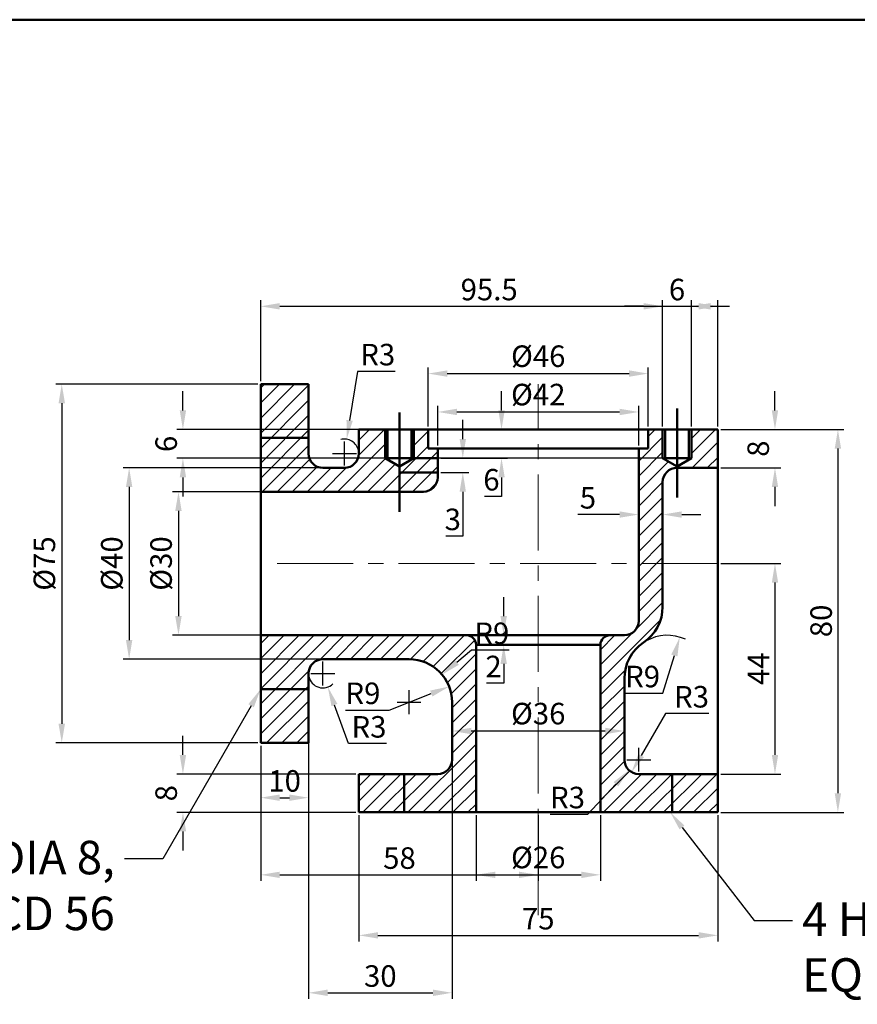
# Model space of a CAD drawing. Units: millimetres. Extents: x -166 to 681, y -4360 to 126.
# Tile 4 of 7: x -22 to 153, y -80 to 126. Entities that reach past the tile are written whole.
import ezdxf
from ezdxf import colors
from ezdxf.entities.mleader import LeaderData, LeaderLine
from ezdxf.math import Vec2, Vec3

# ---------------------------------------------------------------- set-up
doc = ezdxf.new("R2010")
doc.units = ezdxf.units.MM
doc.header["$LTSCALE"] = 0.5
doc.linetypes.add('CENTER', pattern=[50.8, 31.75, -6.35, 6.35, -6.35])
for name, color, linetype, lineweight in [('M-CNTR', 1, 'CENTER', 18), ('M-DIMS', 2, 'Continuous', 25), ('M-HATC', 8, 'Continuous', 18), ('M-OUTL', 7, 'Continuous', 50), ('M-TEXT', 7, 'Continuous', 25), ('M-TTLB', 7, 'Continuous', 50)]:
    doc.layers.add(name, color=color, linetype=linetype, lineweight=lineweight)
doc.styles.get("Standard").update_dxf_attribs({"font": 'arial.ttf'})
doc.dimstyles.new('ISO-25', dxfattribs={"dimtxt": 4.5, "dimasz": 4, "dimexe": 1.25, "dimexo": 0.625, "dimtad": 1, "dimtoh": 1, "dimdec": 1, "dimtxsty": 'Standard', "dimcen": 2.5, "dimadec": 0, "dimazin": 0, "dimtfac": 1, "dimtdec": 1, "dimtofl": 0, "dimtmove": 0, "dimatfit": 3, "dimfxl": 1, "dimarcsym": 0})
pattern_1 = [(45, (-558537.9113, -290104.013), (-1.571544821, 1.571544821), [])]

# ---------------------------------------------------------------- blocks, each defined once
blk = doc.blocks.new('*D1')
at = {"layer": 'Defpoints', "color": 0, "transparency": 16777216}
for p in [(49.3, -39.56), (124.3, -39.56), (124.3, -65.27)]:
    blk.add_point(p, dxfattribs=at)
at = {"layer": 'M-DIMS', "color": 0, "lineweight": -2, "transparency": 16777216}
for p, q in [((49.3, -40.18), (49.3, -66.52)), ((124.3, -40.18), (124.3, -66.52)), ((53.3, -65.27), (120.3, -65.27))]:
    blk.add_line(p, q, dxfattribs=at)
at = {"layer": 'M-DIMS', "color": 0, "transparency": 16777216}
for points in [[(53.3, -64.6), (53.3, -65.94), (49.3, -65.27)], [(120.3, -64.6), (120.3, -65.94), (124.3, -65.27)]]:
    blk.add_solid(points, dxfattribs=at)
at = {"layer": 'M-DIMS', "color": 0, "transparency": 16777216, "insert": (86.8, -62.36), "char_height": 4.5, "attachment_point": 5}
blk.add_mtext('75', dxfattribs=at)
blk = doc.blocks.new('*D2')
at = {"layer": 'Defpoints', "color": 0, "transparency": 16777216}
for p in [(73.8, -39.56), (99.8, -39.56), (99.8, -52.62)]:
    blk.add_point(p, dxfattribs=at)
at = {"layer": 'M-DIMS', "color": 0, "lineweight": -2, "transparency": 16777216}
for p, q in [((73.8, -40.18), (73.8, -53.87)), ((99.8, -40.18), (99.8, -53.87)), ((77.8, -52.62), (95.8, -52.62))]:
    blk.add_line(p, q, dxfattribs=at)
at = {"layer": 'M-DIMS', "color": 0, "transparency": 16777216}
for points in [[(77.8, -51.96), (77.8, -53.29), (73.8, -52.62)], [(95.8, -51.96), (95.8, -53.29), (99.8, -52.62)]]:
    blk.add_solid(points, dxfattribs=at)
at = {"layer": 'M-DIMS', "color": 0, "transparency": 16777216, "insert": (86.8, -49.58), "char_height": 4.5, "attachment_point": 5}
blk.add_mtext('%%C26', dxfattribs=at)
blk = doc.blocks.new('*D3')
at = {"layer": 'Defpoints', "color": 0, "transparency": 16777216}
for p in [(28.8, -25.06), (86.8, -39.56), (86.8, -52.62)]:
    blk.add_point(p, dxfattribs=at)
at = {"layer": 'M-DIMS', "color": 0, "lineweight": -2, "transparency": 16777216}
for p, q in [((28.8, -25.68), (28.8, -53.87)), ((86.8, -40.18), (86.8, -53.87)), ((32.8, -52.62), (82.8, -52.62))]:
    blk.add_line(p, q, dxfattribs=at)
at = {"layer": 'M-DIMS', "color": 0, "transparency": 16777216}
for points in [[(32.8, -51.96), (32.8, -53.29), (28.8, -52.62)], [(82.8, -51.96), (82.8, -53.29), (86.8, -52.62)]]:
    blk.add_solid(points, dxfattribs=at)
at = {"layer": 'M-DIMS', "color": 0, "transparency": 16777216, "insert": (57.8, -49.7), "char_height": 4.5, "attachment_point": 5}
blk.add_mtext('58', dxfattribs=at)
blk = doc.blocks.new('*D4')
at = {"layer": 'Defpoints', "color": 0, "transparency": 16777216}
for p in [(28.8, -25.06), (38.8, -25.06), (38.8, -36.5)]:
    blk.add_point(p, dxfattribs=at)
at = {"layer": 'M-DIMS', "color": 0, "lineweight": -2, "transparency": 16777216}
for p, q in [((28.8, -25.68), (28.8, -37.75)), ((38.8, -25.68), (38.8, -37.75)), ((32.8, -36.5), (34.8, -36.5))]:
    blk.add_line(p, q, dxfattribs=at)
at = {"layer": 'M-DIMS', "color": 0, "transparency": 16777216}
for points in [[(32.8, -35.83), (32.8, -37.17), (28.8, -36.5)], [(34.8, -35.83), (34.8, -37.17), (38.8, -36.5)]]:
    blk.add_solid(points, dxfattribs=at)
at = {"layer": 'M-DIMS', "color": 0, "transparency": 16777216, "insert": (33.8, -33.58), "char_height": 4.5, "attachment_point": 5}
blk.add_mtext('10', dxfattribs=at)
blk = doc.blocks.new('*D5')
at = {"layer": 'Defpoints', "color": 0, "transparency": 16777216}
for p in [(68.8, -22.56), (104.8, -22.56), (104.8, -22.56)]:
    blk.add_point(p, dxfattribs=at)
at = {"layer": 'M-DIMS', "color": 0, "lineweight": -2, "transparency": 16777216}
for p, q in [((68.8, -21.93), (68.8, -21.31)), ((72.8, -22.56), (100.8, -22.56)), ((104.8, -21.93), (104.8, -21.31))]:
    blk.add_line(p, q, dxfattribs=at)
at = {"layer": 'M-DIMS', "color": 0, "transparency": 16777216}
for points in [[(72.8, -21.89), (72.8, -23.23), (68.8, -22.56)], [(100.8, -21.89), (100.8, -23.23), (104.8, -22.56)]]:
    blk.add_solid(points, dxfattribs=at)
at = {"layer": 'M-DIMS', "color": 0, "transparency": 16777216, "insert": (86.8, -19.51), "char_height": 4.5, "attachment_point": 5}
blk.add_mtext('%%C36', dxfattribs=at)
blk = doc.blocks.new('*D6')
at = {"layer": 'Defpoints', "color": 0, "ltscale": 0.5, "transparency": 16777216}
for p in [(28.8, 49.94), (-12.77, -25.06), (28.8, -25.06)]:
    blk.add_point(p, dxfattribs=at)
at = {"layer": 'M-DIMS', "color": 0, "lineweight": -2, "ltscale": 0.5, "transparency": 16777216}
for p, q in [((28.18, 49.94), (-14.02, 49.94)), ((-12.77, 45.94), (-12.77, -21.06)), ((28.18, -25.06), (-14.02, -25.06))]:
    blk.add_line(p, q, dxfattribs=at)
at = {"layer": 'M-DIMS', "color": 0, "ltscale": 0.5, "transparency": 16777216}
for points in [[(-13.44, 45.94), (-12.1, 45.94), (-12.77, 49.94)], [(-13.44, -21.06), (-12.1, -21.06), (-12.77, -25.06)]]:
    blk.add_solid(points, dxfattribs=at)
at = {"layer": 'M-DIMS', "color": 0, "ltscale": 0.5, "transparency": 16777216, "insert": (-15.82, 12.44), "char_height": 4.5, "attachment_point": 5, "rotation": 90}
blk.add_mtext('%%C75', dxfattribs=at)
blk = doc.blocks.new('*D7')
at = {"layer": 'Defpoints', "color": 0, "ltscale": 0.5, "transparency": 16777216}
for p in [(44.05, 32.44), (1.31, -7.56), (44.05, -7.56)]:
    blk.add_point(p, dxfattribs=at)
at = {"layer": 'M-DIMS', "color": 0, "lineweight": -2, "ltscale": 0.5, "transparency": 16777216}
for p, q in [((43.43, 32.44), (0.06, 32.44)), ((1.31, 28.44), (1.31, -3.56)), ((43.43, -7.56), (0.06, -7.56))]:
    blk.add_line(p, q, dxfattribs=at)
at = {"layer": 'M-DIMS', "color": 0, "ltscale": 0.5, "transparency": 16777216}
for points in [[(0.65, 28.44), (1.98, 28.44), (1.31, 32.44)], [(0.65, -3.56), (1.98, -3.56), (1.31, -7.56)]]:
    blk.add_solid(points, dxfattribs=at)
at = {"layer": 'M-DIMS', "color": 0, "ltscale": 0.5, "transparency": 16777216, "insert": (-1.73, 12.44), "char_height": 4.5, "attachment_point": 5, "rotation": 90}
blk.add_mtext('%%C40', dxfattribs=at)
blk = doc.blocks.new('*D8')
at = {"layer": 'Defpoints', "color": 0, "ltscale": 0.5, "transparency": 16777216}
for p in [(45.8, 27.44), (11.62, -2.56), (45.8, -2.56)]:
    blk.add_point(p, dxfattribs=at)
at = {"layer": 'M-DIMS', "color": 0, "lineweight": -2, "ltscale": 0.5, "transparency": 16777216}
for p, q in [((45.18, 27.44), (10.37, 27.44)), ((11.62, 23.44), (11.62, 1.44)), ((45.18, -2.56), (10.37, -2.56))]:
    blk.add_line(p, q, dxfattribs=at)
at = {"layer": 'M-DIMS', "color": 0, "ltscale": 0.5, "transparency": 16777216}
for points in [[(10.95, 23.44), (12.28, 23.44), (11.62, 27.44)], [(10.95, 1.44), (12.28, 1.44), (11.62, -2.56)]]:
    blk.add_solid(points, dxfattribs=at)
at = {"layer": 'M-DIMS', "color": 0, "ltscale": 0.5, "transparency": 16777216, "insert": (8.57, 12.44), "char_height": 4.5, "attachment_point": 5, "rotation": 90}
blk.add_mtext('%%C30', dxfattribs=at)
blk = doc.blocks.new('*D9')
at = {"layer": 'Defpoints', "color": 0, "ltscale": 0.5, "transparency": 16777216}
for p in [(109.8, 52.13), (63.8, 40.44), (109.8, 40.44)]:
    blk.add_point(p, dxfattribs=at)
at = {"layer": 'M-DIMS', "color": 0, "lineweight": -2, "ltscale": 0.5, "transparency": 16777216}
for p, q in [((63.8, 41.07), (63.8, 53.38)), ((67.8, 52.13), (105.8, 52.13)), ((109.8, 41.07), (109.8, 53.38))]:
    blk.add_line(p, q, dxfattribs=at)
at = {"layer": 'M-DIMS', "color": 0, "ltscale": 0.5, "transparency": 16777216}
for points in [[(67.8, 52.8), (67.8, 51.47), (63.8, 52.13)], [(105.8, 52.8), (105.8, 51.47), (109.8, 52.13)]]:
    blk.add_solid(points, dxfattribs=at)
at = {"layer": 'M-DIMS', "color": 0, "ltscale": 0.5, "transparency": 16777216, "insert": (86.8, 55.18), "char_height": 4.5, "attachment_point": 5}
blk.add_mtext('%%C46', dxfattribs=at)
blk = doc.blocks.new('*D10')
at = {"layer": 'Defpoints', "color": 0, "ltscale": 0.5, "transparency": 16777216}
for p in [(107.8, 44.11), (65.8, 36.44), (107.8, 36.44)]:
    blk.add_point(p, dxfattribs=at)
at = {"layer": 'M-DIMS', "color": 0, "lineweight": -2, "ltscale": 0.5, "transparency": 16777216}
for p, q in [((65.8, 37.07), (65.8, 45.36)), ((107.8, 37.07), (107.8, 45.36)), ((69.8, 44.11), (103.8, 44.11))]:
    blk.add_line(p, q, dxfattribs=at)
at = {"layer": 'M-DIMS', "color": 0, "ltscale": 0.5, "transparency": 16777216}
for points in [[(69.8, 44.78), (69.8, 43.44), (65.8, 44.11)], [(103.8, 44.78), (103.8, 43.44), (107.8, 44.11)]]:
    blk.add_solid(points, dxfattribs=at)
at = {"layer": 'M-DIMS', "color": 0, "ltscale": 0.5, "transparency": 16777216, "insert": (86.8, 47.16), "char_height": 4.5, "attachment_point": 5}
blk.add_mtext('%%C42', dxfattribs=at)
blk = doc.blocks.new('*D11')
at = {"layer": 'Defpoints', "color": 0, "ltscale": 0.5, "transparency": 16777216}
for p in [(124.3, 12.44), (124.3, -31.56), (136.27, -31.56)]:
    blk.add_point(p, dxfattribs=at)
at = {"layer": 'M-DIMS', "color": 0, "lineweight": -2, "ltscale": 0.5, "transparency": 16777216}
for p, q in [((124.93, 12.44), (137.52, 12.44)), ((136.27, 8.44), (136.27, -27.56)), ((124.93, -31.56), (137.52, -31.56))]:
    blk.add_line(p, q, dxfattribs=at)
at = {"layer": 'M-DIMS', "color": 0, "ltscale": 0.5, "transparency": 16777216}
for points in [[(135.61, 8.44), (136.94, 8.44), (136.27, 12.44)], [(135.61, -27.56), (136.94, -27.56), (136.27, -31.56)]]:
    blk.add_solid(points, dxfattribs=at)
at = {"layer": 'M-DIMS', "color": 0, "ltscale": 0.5, "transparency": 16777216, "insert": (133.4, -9.56), "char_height": 4.5, "attachment_point": 5, "rotation": 90}
blk.add_mtext('44', dxfattribs=at)
blk = doc.blocks.new('*D12')
at = {"layer": 'Defpoints', "color": 0, "ltscale": 0.5, "transparency": 16777216}
for p in [(124.3, 40.44), (124.3, 32.44), (136.27, 32.44)]:
    blk.add_point(p, dxfattribs=at)
at = {"layer": 'M-DIMS', "color": 0, "lineweight": -2, "ltscale": 0.5, "transparency": 16777216}
for p, q in [((136.27, 44.44), (136.27, 48.44)), ((124.93, 40.44), (137.52, 40.44)), ((124.93, 32.44), (137.52, 32.44)), ((136.27, 28.44), (136.27, 24.44))]:
    blk.add_line(p, q, dxfattribs=at)
at = {"layer": 'M-DIMS', "color": 0, "ltscale": 0.5, "transparency": 16777216}
for points in [[(135.61, 44.44), (136.94, 44.44), (136.27, 40.44)], [(135.61, 28.44), (136.94, 28.44), (136.27, 32.44)]]:
    blk.add_solid(points, dxfattribs=at)
at = {"layer": 'M-DIMS', "color": 0, "ltscale": 0.5, "transparency": 16777216, "insert": (133.35, 36.44), "char_height": 4.5, "attachment_point": 5, "rotation": 90}
blk.add_mtext('8', dxfattribs=at)
blk = doc.blocks.new('*D13')
at = {"layer": 'Defpoints', "color": 0, "ltscale": 0.5, "transparency": 16777216}
for p in [(124.3, 40.44), (124.3, -39.56), (149.42, -39.56)]:
    blk.add_point(p, dxfattribs=at)
at = {"layer": 'M-DIMS', "color": 0, "lineweight": -2, "ltscale": 0.5, "transparency": 16777216}
for p, q in [((124.93, 40.44), (150.67, 40.44)), ((149.42, 36.44), (149.42, -35.56)), ((124.93, -39.56), (150.67, -39.56))]:
    blk.add_line(p, q, dxfattribs=at)
at = {"layer": 'M-DIMS', "color": 0, "ltscale": 0.5, "transparency": 16777216}
for points in [[(148.75, 36.44), (150.09, 36.44), (149.42, 40.44)], [(148.75, -35.56), (150.09, -35.56), (149.42, -39.56)]]:
    blk.add_solid(points, dxfattribs=at)
at = {"layer": 'M-DIMS', "color": 0, "ltscale": 0.5, "transparency": 16777216, "insert": (146.5, 0.44), "char_height": 4.5, "attachment_point": 5, "rotation": 90}
blk.add_mtext('80', dxfattribs=at)
blk = doc.blocks.new('*D14')
at = {"layer": 'Defpoints', "color": 0, "ltscale": 0.5, "transparency": 16777216}
for p in [(112.8, 22.67), (107.8, 22.01), (112.8, 22.01)]:
    blk.add_point(p, dxfattribs=at)
at = {"layer": 'M-DIMS', "color": 0, "lineweight": -2, "ltscale": 0.5, "transparency": 16777216}
for p, q in [((103.8, 22.67), (95.07, 22.67)), ((107.8, 22.63), (107.8, 23.92)), ((112.8, 22.63), (112.8, 23.92)), ((116.8, 22.67), (120.8, 22.67))]:
    blk.add_line(p, q, dxfattribs=at)
at = {"layer": 'M-DIMS', "color": 0, "ltscale": 0.5, "transparency": 16777216}
for points in [[(103.8, 23.34), (103.8, 22.01), (107.8, 22.67)], [(116.8, 23.34), (116.8, 22.01), (112.8, 22.67)]]:
    blk.add_solid(points, dxfattribs=at)
at = {"layer": 'M-DIMS', "color": 0, "ltscale": 0.5, "transparency": 16777216, "insert": (97.19, 25.59), "char_height": 4.5, "attachment_point": 5}
blk.add_mtext('5', dxfattribs=at)
blk = doc.blocks.new('*D15')
at = {"layer": 'Defpoints', "color": 0, "ltscale": 0.5, "transparency": 16777216}
for p in [(65.8, 34.44), (65.8, 31.44), (71.04, 31.44)]:
    blk.add_point(p, dxfattribs=at)
at = {"layer": 'M-DIMS', "color": 0, "lineweight": -2, "ltscale": 0.5, "transparency": 16777216}
for p, q in [((71.04, 38.44), (71.04, 42.44)), ((66.43, 34.44), (72.29, 34.44)), ((66.43, 31.44), (72.29, 31.44)), ((71.04, 27.44), (71.04, 18.16)), ((71.04, 18.16), (67.46, 18.16))]:
    blk.add_line(p, q, dxfattribs=at)
at = {"layer": 'M-DIMS', "color": 0, "ltscale": 0.5, "transparency": 16777216}
for points in [[(70.37, 38.44), (71.7, 38.44), (71.04, 34.44)], [(70.37, 27.44), (71.7, 27.44), (71.04, 31.44)]]:
    blk.add_solid(points, dxfattribs=at)
at = {"layer": 'M-DIMS', "color": 0, "ltscale": 0.5, "transparency": 16777216, "insert": (68.94, 21.08), "char_height": 4.5, "attachment_point": 5}
blk.add_mtext('3', dxfattribs=at)
blk = doc.blocks.new('*D16')
at = {"layer": 'Defpoints', "color": 0, "ltscale": 0.5, "transparency": 16777216}
for p in [(65.8, 40.44), (65.8, 34.44), (79.13, 34.44)]:
    blk.add_point(p, dxfattribs=at)
at = {"layer": 'M-DIMS', "color": 0, "lineweight": -2, "ltscale": 0.5, "transparency": 16777216}
for p, q in [((79.13, 44.44), (79.13, 48.44)), ((66.43, 40.44), (80.38, 40.44)), ((66.43, 34.44), (80.38, 34.44)), ((79.13, 30.44), (79.13, 26.44)), ((79.13, 26.44), (75.54, 26.44))]:
    blk.add_line(p, q, dxfattribs=at)
at = {"layer": 'M-DIMS', "color": 0, "ltscale": 0.5, "transparency": 16777216}
for points in [[(78.47, 44.44), (79.8, 44.44), (79.13, 40.44)], [(78.47, 30.44), (79.8, 30.44), (79.13, 34.44)]]:
    blk.add_solid(points, dxfattribs=at)
at = {"layer": 'M-DIMS', "color": 0, "ltscale": 0.5, "transparency": 16777216, "insert": (77.02, 29.36), "char_height": 4.5, "attachment_point": 5}
blk.add_mtext('6', dxfattribs=at)
blk = doc.blocks.new('*D17')
at = {"layer": 'Defpoints', "color": 0, "ltscale": 0.5, "transparency": 16777216}
for p in [(77.02, -2.56), (77.02, -4.56), (79.58, -4.56)]:
    blk.add_point(p, dxfattribs=at)
at = {"layer": 'M-DIMS', "color": 0, "lineweight": -2, "ltscale": 0.5, "transparency": 16777216}
for p, q in [((79.58, 1.44), (79.58, 5.44)), ((77.65, -2.56), (80.83, -2.56)), ((77.65, -4.56), (80.83, -4.56)), ((79.58, -8.56), (79.58, -12.56)), ((79.58, -12.56), (75.97, -12.56))]:
    blk.add_line(p, q, dxfattribs=at)
at = {"layer": 'M-DIMS', "color": 0, "ltscale": 0.5, "transparency": 16777216}
for points in [[(78.91, 1.44), (80.25, 1.44), (79.58, -2.56)], [(78.91, -8.56), (80.25, -8.56), (79.58, -4.56)]]:
    blk.add_solid(points, dxfattribs=at)
at = {"layer": 'M-DIMS', "color": 0, "ltscale": 0.5, "transparency": 16777216, "insert": (77.46, -9.67), "char_height": 4.5, "attachment_point": 5}
blk.add_mtext('2', dxfattribs=at)
blk = doc.blocks.new('*D18')
at = {"layer": 'Defpoints', "color": 0, "ltscale": 0.5, "transparency": 16777216}
for p in [(41.8, -10.56), (42.83, -13.38)]:
    blk.add_point(p, dxfattribs=at)
at = {"layer": 'M-DIMS', "color": 0, "lineweight": -2, "ltscale": 0.5, "transparency": 16777216}
for p, q in [((41.8, -13.06), (41.8, -8.06)), ((39.3, -10.56), (44.3, -10.56)), ((47.17, -25.2), (44.21, -17.13)), ((55.06, -25.2), (47.17, -25.2))]:
    blk.add_line(p, q, dxfattribs=at)
blk.add_arc((41.8, -10.56), 3, 191.9366, 314.026, dxfattribs=at)
at = {"layer": 'M-DIMS', "color": 0, "ltscale": 0.5, "transparency": 16777216}
blk.add_solid([(44.84, -16.9), (43.59, -17.36), (42.83, -13.38)], dxfattribs=at)
at = {"layer": 'M-DIMS', "color": 0, "ltscale": 0.5, "transparency": 16777216, "insert": (51.43, -22.28), "char_height": 4.5, "attachment_point": 5}
blk.add_mtext('R3', dxfattribs=at)
blk = doc.blocks.new('*D19')
at = {"layer": 'Defpoints', "color": 0, "ltscale": 0.5, "transparency": 16777216}
for p in [(68.18, -13.27), (59.8, -16.56)]:
    blk.add_point(p, dxfattribs=at)
at = {"layer": 'M-DIMS', "color": 0, "lineweight": -2, "ltscale": 0.5, "transparency": 16777216}
for p, q in [((55.64, -18.19), (64.46, -14.73)), ((46.54, -18.19), (55.64, -18.19))]:
    blk.add_line(p, q, dxfattribs=at)
at = {"layer": 'M-DIMS', "color": 0, "ltscale": 0.5, "transparency": 16777216}
blk.add_solid([(64.21, -14.11), (64.7, -15.35), (68.18, -13.27)], dxfattribs=at)
at = {"layer": 'M-DIMS', "color": 0, "ltscale": 0.5, "transparency": 16777216, "insert": (50.17, -15.27), "char_height": 4.5, "attachment_point": 5}
blk.add_mtext('R9', dxfattribs=at)
blk = doc.blocks.new('*D20')
at = {"layer": 'Defpoints', "color": 0, "ltscale": 0.5, "transparency": 16777216}
for p in [(107.8, -28.56), (106.3, -31.16)]:
    blk.add_point(p, dxfattribs=at)
at = {"layer": 'M-DIMS', "color": 0, "lineweight": -2, "ltscale": 0.5, "transparency": 16777216}
for p, q in [((113.37, -18.92), (108.3, -27.69)), ((122.46, -18.92), (113.37, -18.92))]:
    blk.add_line(p, q, dxfattribs=at)
at = {"layer": 'M-DIMS', "color": 0, "ltscale": 0.5, "transparency": 16777216}
blk.add_solid([(107.72, -27.36), (108.88, -28.03), (106.3, -31.16)], dxfattribs=at)
at = {"layer": 'M-DIMS', "color": 0, "ltscale": 0.5, "transparency": 16777216, "insert": (118.83, -15.99), "char_height": 4.5, "attachment_point": 5}
blk.add_mtext('R3', dxfattribs=at)
blk = doc.blocks.new('*D21')
at = {"layer": 'Defpoints', "color": 0, "ltscale": 0.5, "transparency": 16777216}
for p in [(116.39, -2.94), (113.8, -11.56)]:
    blk.add_point(p, dxfattribs=at)
at = {"layer": 'M-DIMS', "color": 0, "lineweight": -2, "ltscale": 0.5, "transparency": 16777216}
for p, q in [((112.86, -14.68), (115.24, -6.77)), ((104.97, -14.68), (112.86, -14.68))]:
    blk.add_line(p, q, dxfattribs=at)
blk.add_arc((113.8, -11.56), 9, 65.3168, 119.7701, dxfattribs=at)
at = {"layer": 'M-DIMS', "color": 0, "ltscale": 0.5, "transparency": 16777216}
blk.add_solid([(114.6, -6.58), (115.88, -6.96), (116.39, -2.94)], dxfattribs=at)
at = {"layer": 'M-DIMS', "color": 0, "ltscale": 0.5, "transparency": 16777216, "insert": (108.61, -11.76), "char_height": 4.5, "attachment_point": 5}
blk.add_mtext('R9', dxfattribs=at)
blk = doc.blocks.new('*D22')
at = {"layer": 'Defpoints', "color": 0, "ltscale": 0.5, "transparency": 16777216}
for p in [(46.77, 38.4), (46.3, 35.44)]:
    blk.add_point(p, dxfattribs=at)
at = {"layer": 'M-DIMS', "color": 0, "lineweight": -2, "ltscale": 0.5, "transparency": 16777216}
for p, q in [((49.01, 52.58), (47.39, 42.36)), ((56.89, 52.58), (49.01, 52.58)), ((46.3, 32.94), (46.3, 37.94)), ((43.8, 35.44), (48.8, 35.44))]:
    blk.add_line(p, q, dxfattribs=at)
blk.add_arc((46.3, 35.44), 3, 11.9366, 104.8944, dxfattribs=at)
at = {"layer": 'M-DIMS', "color": 0, "ltscale": 0.5, "transparency": 16777216}
blk.add_solid([(46.73, 42.46), (48.05, 42.25), (46.77, 38.4)], dxfattribs=at)
at = {"layer": 'M-DIMS', "color": 0, "ltscale": 0.5, "transparency": 16777216, "insert": (53.26, 55.51), "char_height": 4.5, "attachment_point": 5}
blk.add_mtext('R3', dxfattribs=at)
blk = doc.blocks.new('*D74')
at = {"layer": 'Defpoints', "color": 0, "ltscale": 0.5, "transparency": 16777216}
for p in [(124.3, 66.19), (28.8, 49.94), (124.3, 40.44)]:
    blk.add_point(p, dxfattribs=at)
at = {"layer": 'M-DIMS', "color": 0, "lineweight": -2, "ltscale": 0.5, "transparency": 16777216}
for p, q in [((28.8, 50.57), (28.8, 67.44)), ((32.8, 66.19), (120.3, 66.19)), ((124.3, 41.07), (124.3, 67.44))]:
    blk.add_line(p, q, dxfattribs=at)
at = {"layer": 'M-DIMS', "color": 0, "ltscale": 0.5, "transparency": 16777216}
for points in [[(32.8, 66.86), (32.8, 65.52), (28.8, 66.19)], [(120.3, 66.86), (120.3, 65.52), (124.3, 66.19)]]:
    blk.add_solid(points, dxfattribs=at)
at = {"layer": 'M-DIMS', "color": 0, "ltscale": 0.5, "transparency": 16777216, "insert": (76.55, 69.11), "char_height": 4.5, "attachment_point": 5}
blk.add_mtext('95.5', dxfattribs=at)
blk = doc.blocks.new('*D75')
at = {"layer": 'Defpoints', "color": 0, "ltscale": 0.5, "transparency": 16777216}
for p in [(12.55, -31.56), (49.3, -31.56), (49.3, -39.56)]:
    blk.add_point(p, dxfattribs=at)
at = {"layer": 'M-DIMS', "color": 0, "lineweight": -2, "ltscale": 0.5, "transparency": 16777216}
for p, q in [((12.55, -27.56), (12.55, -23.56)), ((48.68, -31.56), (11.3, -31.56)), ((48.68, -39.56), (11.3, -39.56)), ((12.55, -43.56), (12.55, -47.56))]:
    blk.add_line(p, q, dxfattribs=at)
at = {"layer": 'M-DIMS', "color": 0, "ltscale": 0.5, "transparency": 16777216}
for points in [[(11.88, -27.56), (13.22, -27.56), (12.55, -31.56)], [(11.88, -43.56), (13.22, -43.56), (12.55, -39.56)]]:
    blk.add_solid(points, dxfattribs=at)
at = {"layer": 'M-DIMS', "color": 0, "ltscale": 0.5, "transparency": 16777216, "insert": (9.63, -35.56), "char_height": 4.5, "attachment_point": 5, "rotation": 90}
blk.add_mtext('8', dxfattribs=at)
blk = doc.blocks.new('*D76')
at = {"layer": 'Defpoints', "color": 0, "ltscale": 0.5, "transparency": 16777216}
for p in [(118.8, 66.19), (112.8, 40.44), (118.8, 40.44)]:
    blk.add_point(p, dxfattribs=at)
at = {"layer": 'M-DIMS', "color": 0, "lineweight": -2, "ltscale": 0.5, "transparency": 16777216}
for p, q in [((108.8, 66.19), (104.8, 66.19)), ((112.8, 41.07), (112.8, 67.44)), ((118.8, 41.07), (118.8, 67.44)), ((122.8, 66.19), (126.8, 66.19))]:
    blk.add_line(p, q, dxfattribs=at)
at = {"layer": 'M-DIMS', "color": 0, "ltscale": 0.5, "transparency": 16777216}
for points in [[(108.8, 66.86), (108.8, 65.52), (112.8, 66.19)], [(122.8, 66.86), (122.8, 65.52), (118.8, 66.19)]]:
    blk.add_solid(points, dxfattribs=at)
at = {"layer": 'M-DIMS', "color": 0, "ltscale": 0.5, "transparency": 16777216, "insert": (115.8, 69.11), "char_height": 4.5, "attachment_point": 5}
blk.add_mtext('6', dxfattribs=at)
blk = doc.blocks.new('*D77')
at = {"layer": 'Defpoints', "color": 0, "ltscale": 0.5, "transparency": 16777216}
for p in [(118.8, 40.44), (12.55, 34.44), (118.8, 34.44)]:
    blk.add_point(p, dxfattribs=at)
at = {"layer": 'M-DIMS', "color": 0, "lineweight": -2, "ltscale": 0.5, "transparency": 16777216}
for p, q in [((12.55, 44.44), (12.55, 48.44)), ((118.18, 40.44), (11.3, 40.44)), ((118.18, 34.44), (11.3, 34.44)), ((12.55, 30.44), (12.55, 26.44))]:
    blk.add_line(p, q, dxfattribs=at)
at = {"layer": 'M-DIMS', "color": 0, "ltscale": 0.5, "transparency": 16777216}
for points in [[(11.88, 44.44), (13.22, 44.44), (12.55, 40.44)], [(11.88, 30.44), (13.22, 30.44), (12.55, 34.44)]]:
    blk.add_solid(points, dxfattribs=at)
at = {"layer": 'M-DIMS', "color": 0, "ltscale": 0.5, "transparency": 16777216, "insert": (9.63, 37.44), "char_height": 4.5, "attachment_point": 5, "rotation": 90}
blk.add_mtext('6', dxfattribs=at)
blk = doc.blocks.new('*D82')
at = {"layer": 'Defpoints', "color": 0, "ltscale": 0.5, "transparency": 16777216}
for p in [(38.8, -13.81), (68.8, -16.56), (68.8, -77.27)]:
    blk.add_point(p, dxfattribs=at)
at = {"layer": 'M-DIMS', "color": 0, "lineweight": -2, "ltscale": 0.5, "transparency": 16777216}
for p, q in [((38.8, -14.43), (38.8, -78.52)), ((68.8, -17.18), (68.8, -78.52)), ((42.8, -77.27), (64.8, -77.27))]:
    blk.add_line(p, q, dxfattribs=at)
at = {"layer": 'M-DIMS', "color": 0, "ltscale": 0.5, "transparency": 16777216}
for points in [[(42.8, -76.6), (42.8, -77.94), (38.8, -77.27)], [(64.8, -76.6), (64.8, -77.94), (68.8, -77.27)]]:
    blk.add_solid(points, dxfattribs=at)
at = {"layer": 'M-DIMS', "color": 0, "ltscale": 0.5, "transparency": 16777216, "insert": (53.8, -74.35), "char_height": 4.5, "attachment_point": 5}
blk.add_mtext('30', dxfattribs=at)
blk = doc.blocks.new('*D92')
at = {"layer": 'Defpoints', "color": 0, "ltscale": 0.5, "transparency": 16777216}
for p in [(66.7, -10.78), (59.8, -16.56)]:
    blk.add_point(p, dxfattribs=at)
at = {"layer": 'M-DIMS', "color": 0, "lineweight": -2, "ltscale": 0.5, "transparency": 16777216}
for p, q in [((72.84, -5.65), (69.77, -8.22)), ((80.73, -5.65), (72.84, -5.65)), ((59.8, -19.06), (59.8, -14.06)), ((57.3, -16.56), (62.3, -16.56))]:
    blk.add_line(p, q, dxfattribs=at)
at = {"layer": 'M-DIMS', "color": 0, "ltscale": 0.5, "transparency": 16777216}
blk.add_solid([(69.34, -7.7), (70.2, -8.73), (66.7, -10.78)], dxfattribs=at)
at = {"layer": 'M-DIMS', "color": 0, "ltscale": 0.5, "transparency": 16777216, "insert": (77.1, -2.73), "char_height": 4.5, "attachment_point": 5}
blk.add_mtext('R9', dxfattribs=at)
blk = doc.blocks.new('*D93')
at = {"layer": 'Defpoints', "color": 0, "ltscale": 0.5, "transparency": 16777216}
for p in [(107.8, -28.56), (105.76, -30.75)]:
    blk.add_point(p, dxfattribs=at)
at = {"layer": 'M-DIMS', "color": 0, "lineweight": -2, "ltscale": 0.5, "transparency": 16777216}
for p, q in [((107.8, -31.06), (107.8, -26.06)), ((105.3, -28.56), (110.3, -28.56)), ((97.17, -39.97), (103.03, -33.68)), ((89.29, -39.97), (97.17, -39.97))]:
    blk.add_line(p, q, dxfattribs=at)
at = {"layer": 'M-DIMS', "color": 0, "ltscale": 0.5, "transparency": 16777216}
blk.add_solid([(102.54, -33.23), (103.52, -34.14), (105.76, -30.75)], dxfattribs=at)
at = {"layer": 'M-DIMS', "color": 0, "ltscale": 0.5, "transparency": 16777216, "insert": (92.92, -37.05), "char_height": 4.5, "attachment_point": 5}
blk.add_mtext('R3', dxfattribs=at)

msp = doc.modelspace()

# ---------------------------------------------------------------- hatches: boundary and pattern name
at = {"layer": 'M-HATC', "ltscale": 0.5}
h = msp.add_hatch(dxfattribs=at)
h.set_pattern_fill('ANSI31', color=256, scale=0.7)
h.set_pattern_definition(pattern_1)
h.paths.add_polyline_path([(38.8008, 49.9412), (28.8008, 49.9412), (28.8008, 38.6912), (38.8008, 38.6912)])
h.paths.add_polyline_path([(57.8008, 32.7092), (54.8008, 34.4412), (54.8008, 40.4412), (49.3008, 40.4412), (49.3008, 35.4412, -0.41421356), (46.3008, 32.4412), (41.8008, 32.4412, -0.41421356), (38.8008, 35.4412), (38.8008, 38.6912), (28.8008, 38.6912), (28.8008, 27.4412), (57.8008, 27.4412)])
h.paths.add_polyline_path([(65.8008, 34.4412), (60.8008, 34.4412), (57.8008, 32.7092), (57.8008, 31.4412), (65.8008, 31.4412)])
h.paths.add_polyline_path([(65.8008, 30.4412), (65.8008, 31.4412), (57.8008, 31.4412), (57.8008, 27.4412), (62.8008, 27.4412, 0.41421356)])
h.paths.add_polyline_path([(124.3008, 40.4412), (118.8008, 40.4412), (118.8008, 34.4412), (115.8008, 32.7092), (115.8008, 32.4412), (124.3008, 32.4412)])
h.paths.add_polyline_path([(115.8008, 32.7092), (112.8008, 34.4412), (112.8008, 40.4412), (109.8008, 40.4412), (109.8008, 36.4412), (107.8008, 36.4412), (107.8008, 12.4412), (112.8008, 12.4412), (112.8008, 29.4412, -0.41421356), (115.8008, 32.4412)])
h.paths.add_polyline_path([(112.8008, 12.4412), (107.8008, 12.4412), (107.8008, 0.4412, -0.41421356), (104.8008, -2.5588), (101.8008, -2.5588, 0.41421356), (99.8008, -4.5588), (99.8008, -39.5588), (124.3008, -39.5588), (124.3008, -31.5588), (107.8008, -31.5588, -0.41421356), (104.8008, -28.5588), (104.8008, -11.5588, -0.25049165), (108.8008, -4.0754, 0.25049165), (112.8008, 3.4079)])
h.paths.add_polyline_path([(73.8008, -4.5588, 0.41421356), (71.8008, -2.5588), (28.8008, -2.5588), (28.8008, -13.8088), (38.8008, -13.8088), (38.8008, -10.5588, -0.41421356), (41.8008, -7.5588), (59.8008, -7.5588, -0.41421356), (68.8008, -16.5588), (68.8008, -28.5588, -0.41421356), (65.8008, -31.5588), (49.3008, -31.5588), (49.3008, -39.5588), (73.8008, -39.5588)])
h.paths.add_polyline_path([(38.8008, -13.8088), (28.8008, -13.8088), (28.8008, -25.0588), (38.8008, -25.0588)], flags=17)
h = msp.add_hatch(dxfattribs=at)
h.set_pattern_fill('ANSI31', color=256, scale=0.7)
h.set_pattern_definition(pattern_1)
h.paths.add_polyline_path([(63.8008, 40.4412), (60.8008, 40.4412), (60.8008, 34.4412), (65.8008, 34.4412), (65.8008, 36.4412), (63.8008, 36.4412)])

# ---------------------------------------------------------------- linework, layer by layer
at = {"layer": 'M-CNTR'}
for p, q in [((86.8008, -61.0209), (86.8008, 49.9412)), ((124.3008, 12.4412), (28.8008, 12.4412))]:
    msp.add_line(p, q, dxfattribs=at)
at = {"layer": 'M-OUTL'}
for p, q in [((38.8008, 49.9412), (28.8008, 49.9412)), ((28.8008, 27.4412), (28.8008, 49.9412)), ((38.8008, 35.4412), (38.8008, 49.9412)), ((57.8008, 43.9754), (57.8008, 23.2561)), ((115.8008, 44.8622), (115.8008, 26.2478)), ((49.3008, 35.4412), (49.3008, 40.4412)), ((109.8008, 40.4412), (49.3008, 40.4412)), ((54.8008, 40.4412), (54.8008, 34.4412)), ((55.3008, 40.4412), (55.3008, 34.1526)), ((60.3008, 40.4412), (60.3008, 34.1526)), ((60.8008, 40.4412), (60.8008, 34.4412)), ((63.8008, 36.4412), (63.8008, 40.4412)), ((115.8008, 40.4412), (109.8008, 40.4412)), ((109.8008, 36.4412), (109.8008, 40.4412)), ((112.8008, 40.4412), (112.8008, 34.4412)), ((113.3008, 40.4412), (113.3008, 34.1526)), ((124.3008, 40.4412), (115.8008, 40.4412)), ((118.3008, 40.4412), (118.3008, 34.1526)), ((118.8008, 40.4412), (118.8008, 34.4412)), ((124.3008, -31.5588), (124.3008, 40.4412)), ((28.8008, 38.6912), (38.8008, 38.6912)), ((109.8008, 36.4412), (63.8008, 36.4412)), ((65.8008, 30.4412), (65.8008, 36.4412)), ((107.8008, 0.4412), (107.8008, 36.4412)), ((57.8008, 32.7092), (54.8008, 34.4412)), ((60.3008, 34.4412), (55.3008, 34.4412)), ((60.8008, 34.4412), (57.8008, 32.7092)), ((65.8008, 34.4412), (60.8008, 34.4412)), ((112.8008, 34.4412), (115.8008, 32.7092)), ((118.3008, 34.4412), (113.3008, 34.4412)), ((115.8008, 32.7092), (118.8008, 34.4412)), ((46.3008, 32.4412), (41.8008, 32.4412)), ((65.8008, 31.4412), (57.8008, 31.4412)), ((124.3008, 32.4412), (115.8008, 32.4412)), ((112.8008, 3.4079), (112.8008, 29.4412)), ((28.8008, -25.0588), (28.8008, 27.4412)), ((62.8008, 27.4412), (28.8008, 27.4412)), ((71.8008, -2.5588), (28.8008, -2.5588)), ((71.8008, -2.5588), (101.8008, -2.5588)), ((104.8008, -2.5588), (101.8008, -2.5588)), ((73.8008, -39.5588), (73.8008, -4.5588)), ((73.8008, -4.5588), (99.8008, -4.5588)), ((99.8008, -39.5588), (99.8008, -4.5588)), ((59.8008, -7.5588), (41.8008, -7.5588)), ((38.8008, -25.0588), (38.8008, -10.5588)), ((104.8008, -28.5588), (104.8008, -11.5588)), ((28.8008, -13.8088), (38.8008, -13.8088)), ((68.8008, -28.5588), (68.8008, -16.5588)), ((38.8008, -25.0588), (28.8008, -25.0588)), ((49.3008, -31.5588), (49.3008, -39.5588)), ((65.8008, -31.5588), (49.3008, -31.5588)), ((124.3008, -31.5588), (107.8008, -31.5588)), ((124.3008, -39.5588), (124.3008, -31.5588)), ((49.3008, -39.5588), (124.3008, -39.5588))]:
    msp.add_line(p, q, dxfattribs=at)
at = {"layer": 'M-OUTL', "ltscale": 0.5}
for p, q in [((58.8008, -39.5588), (58.8008, -31.5588)), ((114.8008, -39.5588), (114.8008, -31.5588))]:
    msp.add_line(p, q, dxfattribs=at)
at = {"layer": 'M-OUTL'}
for centre, radius, start, end in [((41.8008, 35.4412), 3, 180, 270), ((46.3008, 35.4412), 3, 270, 0), ((115.8008, 29.4412), 3, 90, 180), ((62.8008, 30.4412), 3, 270, 0), ((103.8008, 3.4079), 9, 303.748989, 0), ((104.8008, 0.4412), 3, 270, 0), ((71.8008, -4.5588), 2, 0, 90), ((101.8008, -4.5588), 2, 90, 180), ((113.8008, -11.5588), 9, 123.748989, 180), ((41.8008, -10.5588), 3, 90, 180), ((59.8008, -16.5588), 9, 0, 90), ((65.8008, -28.5588), 3, 270, 0), ((107.8008, -28.5588), 3, 180, 270)]:
    msp.add_arc(centre, radius, start, end, dxfattribs=at)
at = {"layer": 'M-TTLB', "ltscale": 0.5}
msp.add_lwpolyline([(-165.9437, 126.0872), (680.7907, 126.0872), (680.7907, -430.0081), (-165.9437, -430.0081)], close=True, dxfattribs=at)

# ---------------------------------------------------------------- dimensions: what is measured, and where the dimension line sits
at = {"layer": 'M-DIMS', "ltscale": 0.5}
for base, p1, p2, override, picture, middle in [((124.3008, 66.1912), (28.8008, 49.9412), (124.3008, 40.4412), {"dimdec": 1, "dimlfac": 1, "dimrnd": 0, "dimzin": 0, "dimdsep": 46, "dimlunit": 2}, '*D74', (76.5508, 69.1138)), ((118.8008, 66.1912), (112.8008, 40.4412), (118.8008, 40.4412), {"dimdec": 0, "dimlfac": 1, "dimrnd": 0, "dimzin": 0, "dimdsep": 46, "dimlunit": 2}, '*D76', (115.8008, 69.1138)), ((68.8008, -77.2709), (38.8008, -13.8088), (68.8008, -16.5588), {"dimdec": 0, "dimlfac": 1, "dimrnd": 0, "dimzin": 0, "dimdsep": 46, "dimlunit": 2}, '*D82', (53.8008, -74.3467))]:
    dim = msp.add_linear_dim(base=base, p1=p1, p2=p2, dimstyle='ISO-25', override=override, dxfattribs=at)
    dim.commit()
    dim.dimension.update_dxf_attribs({"geometry": picture, "text_midpoint": middle})
for center, mpoint, picture, middle in [((46.3008, 35.4412), (46.769, 38.4045), '*D22', (53.2623, 52.5816)), ((113.8008, -11.5588), (116.3909, -2.9395), '*D21', (108.6054, -14.6788)), ((59.8008, -16.5588), (68.1801, -13.2744), '*D19', (50.1714, -18.1895)), ((107.8008, -28.5588), (106.3008, -31.1568), '*D20', (118.829, -18.9191))]:
    dim = msp.add_radius_dim(center=center, mpoint=mpoint, dimstyle='ISO-25', override={"dimclrd": 0, "dimclre": 0, "dimclrt": 0}, dxfattribs=at)
    dim.commit()
    dim.dimension.update_dxf_attribs({"geometry": picture, "text_midpoint": middle, "dimtype": 164})
for base, p1, p2, picture, middle in [((109.8008, 52.1339), (63.8008, 40.4412), (109.8008, 40.4412), '*D9', (86.8008, 55.1823)), ((107.8008, 44.1105), (65.8008, 36.4412), (107.8008, 36.4412), '*D10', (86.8008, 47.1589))]:
    dim = msp.add_linear_dim(base=base, p1=p1, p2=p2, text='%%C<>', dimstyle='ISO-25', override={"dimclrd": 0, "dimclre": 0, "dimclrt": 0}, dxfattribs=at)
    dim.commit()
    dim.dimension.update_dxf_attribs({"geometry": picture, "text_midpoint": middle})
for base, p1, p2, picture, middle in [((-12.7702, -25.0588), (28.8008, 49.9412), (28.8008, -25.0588), '*D6', (-15.8186, 12.4412)), ((1.3147, -7.5588), (44.0508, 32.4412), (44.0508, -7.5588), '*D7', (-1.7338, 12.4412)), ((11.6155, -2.5588), (45.8008, 27.4412), (45.8008, -2.5588), '*D8', (8.5671, 12.4412))]:
    dim = msp.add_linear_dim(base=base, p1=p1, p2=p2, angle=90, text='%%C<>', dimstyle='ISO-25', override={"dimclrd": 0, "dimclre": 0, "dimclrt": 0}, dxfattribs=at)
    dim.commit()
    dim.dimension.update_dxf_attribs({"geometry": picture, "text_midpoint": middle})
for base, p1, p2, override, picture, middle in [((12.5508, 34.4412), (118.8008, 40.4412), (118.8008, 34.4412), {"dimdec": 0, "dimlfac": 1, "dimrnd": 0, "dimzin": 0, "dimdsep": 46, "dimlunit": 2}, '*D77', (9.6282, 37.4412)), ((136.2737, 32.4412), (124.3008, 40.4412), (124.3008, 32.4412), {"dimclrd": 0, "dimclre": 0, "dimclrt": 0}, '*D12', (133.3511, 36.4412)), ((149.4187, -39.5588), (124.3008, 40.4412), (124.3008, -39.5588), {"dimclrd": 0, "dimclre": 0, "dimclrt": 0}, '*D13', (146.4962, 0.4412)), ((136.2737, -31.5588), (124.3008, 12.4412), (124.3008, -31.5588), {"dimclrd": 0, "dimclre": 0, "dimclrt": 0}, '*D11', (133.3987, -9.5588)), ((79.5797, -4.5588), (77.0242, -2.5588), (77.0242, -4.5588), {"dimclrd": 0, "dimclre": 0, "dimclrt": 0}, '*D17', (77.4644, -9.6746)), ((12.5508, -31.5588), (49.3008, -39.5588), (49.3008, -31.5588), {"dimdec": 0, "dimlfac": 1, "dimrnd": 0, "dimzin": 0, "dimdsep": 46, "dimlunit": 2}, '*D75', (9.6282, -35.5588))]:
    dim = msp.add_linear_dim(base=base, p1=p1, p2=p2, angle=90, dimstyle='ISO-25', override=override, dxfattribs=at)
    dim.commit()
    dim.dimension.update_dxf_attribs({"geometry": picture, "text_midpoint": middle})
for base, p1, p2, picture, middle in [((79.1349, 34.4412), (65.8008, 40.4412), (65.8008, 34.4412), '*D16', (77.0242, 26.4412)), ((71.0358, 31.4412), (65.8008, 34.4412), (65.8008, 31.4412), '*D15', (68.9374, 18.1573))]:
    dim = msp.add_linear_dim(base=base, p1=p1, p2=p2, angle=90, dimstyle='ISO-25', override={"dimclrd": 0, "dimclre": 0, "dimclrt": 0}, dxfattribs=at)
    dim.commit()
    dim.dimension.update_dxf_attribs({"geometry": picture, "text_midpoint": middle, "dimtype": 160})
dim = msp.add_linear_dim(base=(112.8008, 22.6723), p1=(107.8008, 22.0056), p2=(112.8008, 22.0056), dimstyle='ISO-25', override={"dimclrd": 0, "dimclre": 0, "dimclrt": 0}, dxfattribs=at)
dim.commit()
dim.dimension.update_dxf_attribs({"geometry": '*D14', "text_midpoint": (97.1867, 22.6723), "dimtype": 160})
for center, mpoint, override, picture, middle in [((59.8008, -16.5588), (66.7031, -10.7831), {"dimdec": 0, "dimlfac": 1, "dimrnd": 0, "dimzin": 0, "dimdsep": 46, "dimlunit": 2}, '*D92', (77.0964, -2.7266)), ((41.8008, -10.5588), (42.8344, -13.3751), {"dimclrd": 0, "dimclre": 0, "dimclrt": 0}, '*D18', (51.428, -22.2779)), ((107.8008, -28.5588), (105.7564, -30.7543), {"dimdec": 0, "dimlfac": 1, "dimrnd": 0, "dimzin": 0, "dimdsep": 46, "dimlunit": 2}, '*D93', (92.9176, -37.0499))]:
    dim = msp.add_radius_dim(center=center, mpoint=mpoint, dimstyle='ISO-25', override=override, dxfattribs=at)
    dim.commit()
    dim.dimension.update_dxf_attribs({"geometry": picture, "text_midpoint": middle})
at = {"layer": 'M-DIMS'}
for base, p1, p2, picture, middle in [((104.8008, -22.5588), (68.8008, -22.5588), (104.8008, -22.5588), '*D5', (86.8008, -19.5103)), ((99.8008, -52.6239), (73.8008, -39.5588), (99.8008, -39.5588), '*D2', (86.8008, -49.5754))]:
    dim = msp.add_linear_dim(base=base, p1=p1, p2=p2, text='%%C<>', dimstyle='ISO-25', override={"dimclrd": 0, "dimclre": 0, "dimclrt": 0}, dxfattribs=at)
    dim.commit()
    dim.dimension.update_dxf_attribs({"geometry": picture, "text_midpoint": middle})
for base, p1, p2, picture, middle in [((86.8008, -52.6239), (28.8008, -25.0588), (86.8008, -39.5588), '*D3', (57.8008, -49.7013)), ((124.3008, -65.2687), (49.3008, -39.5588), (124.3008, -39.5588), '*D1', (86.8008, -62.3554))]:
    dim = msp.add_linear_dim(base=base, p1=p1, p2=p2, dimstyle='ISO-25', override={"dimclrd": 0, "dimclre": 0, "dimclrt": 0}, dxfattribs=at)
    dim.commit()
    dim.dimension.update_dxf_attribs({"geometry": picture, "text_midpoint": middle})
dim = msp.add_linear_dim(base=(38.8008, -36.5008), p1=(28.8008, -25.0588), p2=(38.8008, -25.0588), dimstyle='ISO-25', override={"dimclrd": 0, "dimclre": 0, "dimclrt": 0}, dxfattribs=at)
dim.commit()
dim.dimension.update_dxf_attribs({"geometry": '*D4', "text_midpoint": (33.8008, -36.5008), "dimtype": 160})

# ---------------------------------------------------------------- leaders
at = {"layer": 'M-TEXT', "ltscale": 0.5}
ml = msp.add_multileader_mtext('Standard', dxfattribs=at)
ml.set_content('4 HOLES DIA 8,\\P EQI SP  PCD 56', color=256)
ml.set_leader_properties()
ml.build(insert=Vec2(0, 0))
ctx = ml.context
ctx.base_point, ctx.char_height, ctx.plane_origin = Vec3(-78.2306, -49.2827), 7, Vec3(28.8008, -13.8088)
ctx.text_align_type = 2
notes = []
notes.append((ctx, [(0, (1, 1, 0), (8.3199, -49.2827), (-1, 0), 8, [(0, [(28.8008, -13.8088)], 0, [])])]))
ctx.mtext.insert, ctx.mtext.alignment, ctx.mtext.flow_direction = Vec3(-1.6801, -45.5106), 3, 5
ml = msp.add_multileader_mtext('Standard', dxfattribs=at)
ml.set_content('4 HOLES DIA 8,\\P EQI SP  PCD 56', color=256)
ml.set_leader_properties()
ml.build(insert=Vec2(0, 0))
ctx = ml.context
ctx.base_point, ctx.char_height, ctx.plane_origin = Vec3(139.9432, -62.1565), 7, Vec3(114.3904, -39.5588)
notes.append((ctx, [(1, (1, 1, 0), (131.9432, -62.1565), (1, 0), 8, [(0, [(114.3904, -39.5588)], 0, [])])]))
ctx.mtext.insert, ctx.mtext.flow_direction = Vec3(141.9432, -58.3843), 5
for ctx, leaders in notes:
    for number, flags, end, landing, length, lines in leaders:
        leader = LeaderData()
        leader.index, (leader.has_last_leader_line, leader.has_dogleg_vector, leader.attachment_direction) = number, flags
        leader.last_leader_point, leader.dogleg_vector, leader.dogleg_length = Vec3(end), Vec3(landing), length
        for number, points, colour, breaks in lines:
            line = LeaderLine()
            line.index, line.vertices, line.color, line.breaks = number, Vec3.list(points), colors.encode_raw_color(colour), breaks
            leader.lines.append(line)
        ctx.leaders.append(leader)

doc.saveas('drawing.dxf')
